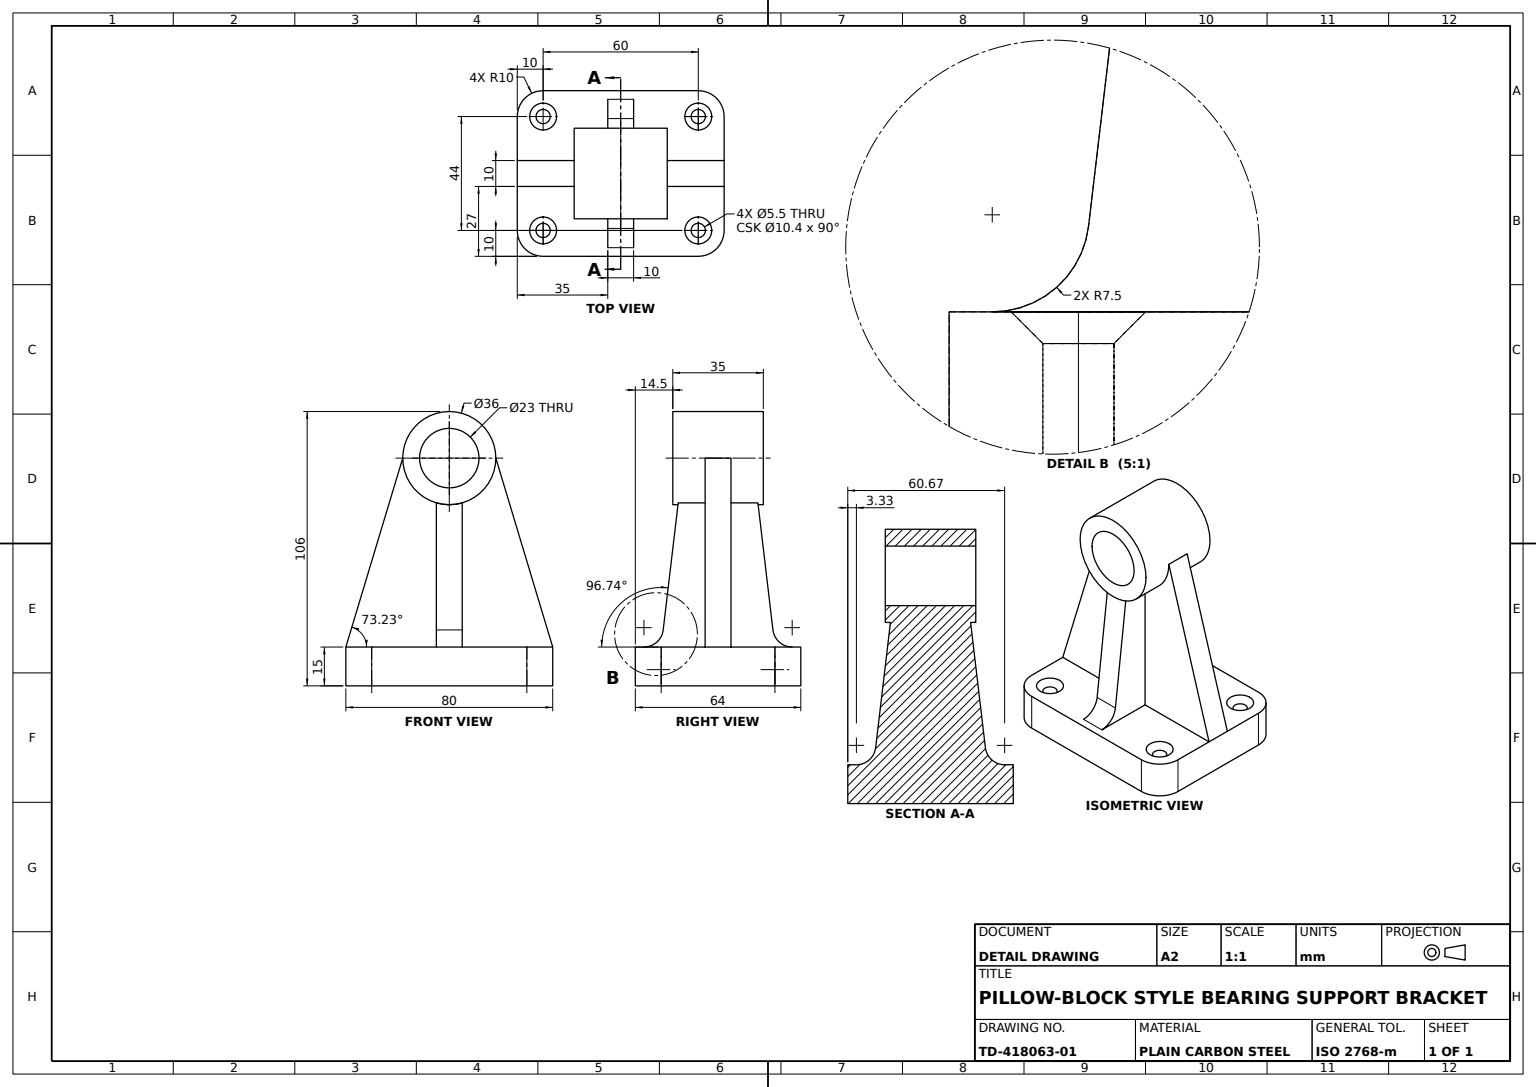
from build123d import *

# Parameters (mm, degrees)
BASE_PLATE_DEPTH                        = 15
BEARING_BOSS_SKETCH_R                   = 18
BEARING_BOSS_SKETCH_R_2                 = 11.5
BEARING_BOSS_36_BORE_23_DEPTH           = 17.5
UPRIGHT_WEB_DEPTH                       = 5
MOUNTING_HOLES_M5_CSK_D                 = 5.5
MOUNTING_HOLES_M5_CSK_CSINK_D           = 10.4
MOUNTING_HOLES_M5_CSK_CSINK_ANGLE       = 90
SUPPORT_RIB_REACH                       = 119.729
SUPPORT_RIB_SKETCH_WALL_W               = 292.839761494
SUPPORT_RIB_SKETCH_WALL_H               = 10
RIB_FILLET_R7_5_R                       = 7.5
RIB_FILLET_R7_5_OF_SUPPORT_RIB_MIRROR_R = 7.5


with BuildPart() as part:
    # Base Plate Sketch → Base Plate (new body)
    with BuildSketch(Plane(origin=(0, 0, 0), x_dir=(1, 0, 0), z_dir=(0, 1, 0))):
        with BuildLine():
            Line((40, 0), (40, 22))
            ThreePointArc((40, 22), (37.071067812, 29.071067812), (30, 32))
            Line((30, 32), (-30, 32))
            ThreePointArc((-30, 32), (-37.071067812, 29.071067812), (-40, 22))
            Line((-40, 22), (-40, -22))
            ThreePointArc((-40, -22), (-37.071067812, -29.071067812), (-30, -32))
            Line((-30, -32), (30, -32))
            ThreePointArc((30, -32), (37.071067812, -29.071067812), (40, -22))
            Line((40, -22), (40, 0))
        make_face()
    extrude(amount=BASE_PLATE_DEPTH)



with BuildPart() as body_2:
    # Bearing Boss Sketch → Bearing Boss Ø36 Bore Ø23 (new, symmetric)
    with BuildSketch(Plane.XY):
        with Locations((0, 88)):
            Circle(BEARING_BOSS_SKETCH_R)
        with Locations((0, 88)):
            Circle(BEARING_BOSS_SKETCH_R_2, mode=Mode.SUBTRACT)
    extrude(amount=BEARING_BOSS_36_BORE_23_DEPTH, both=True)


with BuildPart() as part_1:
    add(part.part)

    add(body_2.part)  # Upright Web merges body 2
    # Upright Web Sketch → Upright Web (add, symmetric)
    with BuildSketch(Plane.XY):
        with BuildLine():
            Line((18, 88), (40, 15))
            Line((40, 15), (-40, 15))
            Line((-40, 15), (-18, 88))
            ThreePointArc((-18, 88), (0, 70), (18, 88))
        make_face()
    extrude(amount=UPRIGHT_WEB_DEPTH, both=True)

    # Mounting Holes M5 CSK (through all)
    with Locations(Plane(origin=(0, 15, 0), x_dir=(1, 0, 0), z_dir=(0, 1, 0))):
        with Locations((-30, 22), (30, 22), (30, -22), (-30, -22)):
            CounterSinkHole(MOUNTING_HOLES_M5_CSK_D / 2, MOUNTING_HOLES_M5_CSK_CSINK_D / 2, counter_sink_angle=MOUNTING_HOLES_M5_CSK_CSINK_ANGLE)

    # Support Rib Sketch wall → Support Rib (add, up to next)
    with BuildSketch(Plane(origin=(0, 42.5, -18.75), x_dir=(0, -0.993088841064, -0.117365044853), z_dir=(0, 0.117365044853, -0.993088841064)), mode=Mode.PRIVATE) as support_rib_sk1:
        Rectangle(SUPPORT_RIB_SKETCH_WALL_W, SUPPORT_RIB_SKETCH_WALL_H)
    support_rib_tool1 = extrude(support_rib_sk1.sketch, amount=-SUPPORT_RIB_REACH, mode=Mode.PRIVATE) - part_1.part
    support_rib = support_rib_tool1.solids().sort_by_distance((0, 42.5, -18.75))[0]
    add(support_rib)

    # Rib Fillet R7.5
    rib_fillet_r7_5_edges = [part_1.edges().sort_by_distance(p)[0] for p in [
        (0, 15, -22),
    ]]
    fillet(rib_fillet_r7_5_edges, radius=RIB_FILLET_R7_5_R)

    # Support Rib Mirror: Support Rib across plane
    add(support_rib.mirror(Plane.XY))

    # Rib Fillet R7.5 of Support Rib Mirror
    rib_fillet_r7_5_of_support_rib_mirror_edges = [part_1.edges().sort_by_distance(p)[0] for p in [
        (0, 15, 22),
    ]]
    fillet(rib_fillet_r7_5_of_support_rib_mirror_edges, radius=RIB_FILLET_R7_5_OF_SUPPORT_RIB_MIRROR_R)


solid = part_1.part
